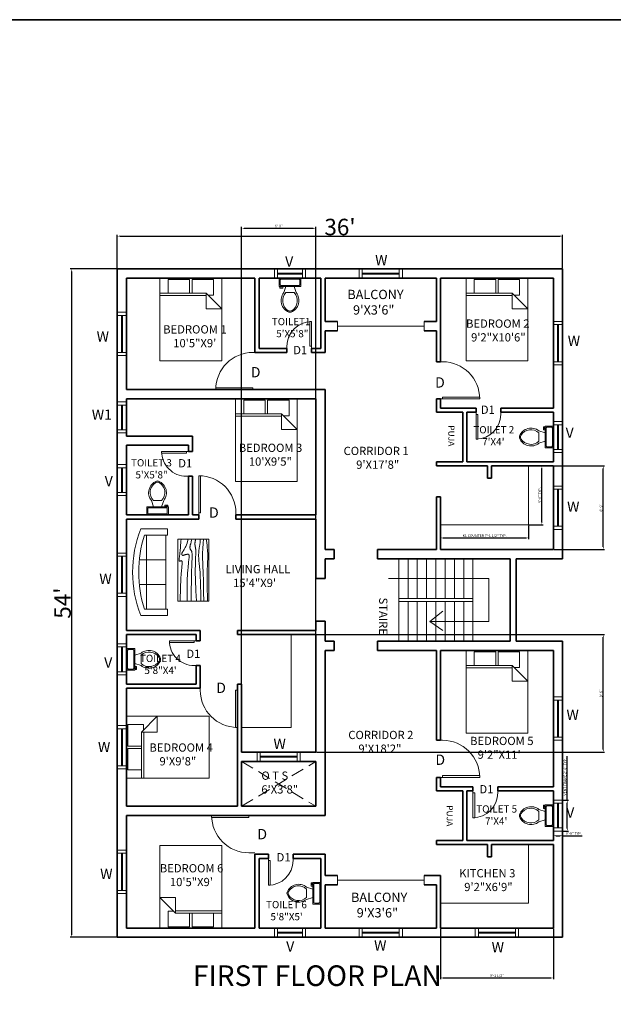
# Model space of a CAD drawing. Units: inches. Extents: x 2391 to 16591, y 7259 to 10239.
# Tile 20 of 27: x 2970 to 3545, y 9285 to 10239. Entities that reach past the tile are written whole.
import ezdxf

# ---------------------------------------------------------------- set-up
doc = ezdxf.new("R2010")
doc.units = ezdxf.units.IN
doc.linetypes.add('DASHED', pattern=[19.05, 12.7, -6.35])
for name, color, linetype, lineweight in [('A-ANNO-DIMS', 4, 'Continuous', 18), ('A-ANNO-IDEN', 2, 'Continuous', 18), ('A-ANNO-SYMB', 3, 'Continuous', 18), ('A-ANNO-TITL', 3, 'Continuous', 30), ('A-ANNO-TTLB', 7, 'Continuous', 35), ('A-AREA-IDEN', 7, 'Continuous', 18), ('A-DOOR', 3, 'Continuous', 18), ('A-FLOR-CASE', 6, 'Continuous', 18), ('A-FLOR-FIXT', 9, 'Continuous', 18), ('A-FLOR-HRAL', 8, 'Continuous', 18), ('A-FLOR-OPEN', 4, 'DASHED', 13), ('A-FLOR-STRS', 7, 'Continuous', 18), ('A-FURN', 8, 'Continuous', 18), ('A-GLAZ', 4, 'Continuous', 18), ('A-WALL', 7, 'Continuous', 35)]:
    doc.layers.add(name, color=color, linetype=linetype, lineweight=lineweight)
doc.styles.get("Standard").update_dxf_attribs({"font": 'arial.ttf'})
doc.dimstyles.new('ISO-25', dxfattribs={"dimtxt": 2.5, "dimasz": 2.5, "dimexe": 1.25, "dimexo": 0.625, "dimtad": 1, "dimdec": 0, "dimlunit": 3, "dimtxsty": 'Standard', "dimcen": 2.5, "dimadec": 0, "dimazin": 0, "dimtfac": 1, "dimtdec": 0, "dimtmove": 0, "dimatfit": 3, "dimfxl": 1, "dimarcsym": 0})

# ---------------------------------------------------------------- blocks, each defined once
blk = doc.blocks.new('Bed - Queen')
for p, q in [((0, -80.00003), (0, 0)), ((0, 0), (59.99999, 0)), ((59.99999, 0), (59.99999, -80.00003)), ((7.99999, -1.2), (28.79998, -1.2)), ((7.99999, -14.4), (7.99999, -1.2)), ((28.79998, -1.2), (28.79998, -14.4)), ((31.19999, -1.2), (51.99999, -1.2)), ((31.19999, -14.4), (31.19999, -1.2)), ((51.99999, -1.2), (51.99999, -16.4)), ((0, -14.4), (44.8, -14.4)), ((44.8, -16.8), (0, -16.8)), ((59.99999, -29.6), (44.8, -14.4)), ((44.8, -14.4), (44.8, -29.6)), ((51.99999, -16.4), (46.79936, -16.4)), ((44.8, -29.6), (59.99999, -29.6)), ((59.99999, -80.00003), (0, -80.00003))]:
    blk.add_line(p, q)
blk = doc.blocks.new('Sofa - Roundback 7 ft.')
for p, q in [((-12.00002, -32.4421), (-12.00003, -6.5971)), ((11.99997, -32.4421), (11.99998, -6.5971)), ((-36.000027, -34), (-36.000027, -11.4696)), ((-35.999844, -13.3819), (35.9998, -13.3819)), ((35.99998, -34), (35.99998, -11.4696)), ((-36.000027, -32.4421), (35.99998, -32.4421))]:
    blk.add_line(p, q)
for points in [[(-36.000027, -34), (-42.000027, -34), (-42.000027, -8)], [(41.99998, -8), (41.99998, -34), (35.99998, -34)]]:
    blk.add_lwpolyline(points)
for centre, radius, start, end in [((0, -114.25), 114.25, 68.43141, 111.5686), ((-0.00001, -127.1968), 121.1968, 72.72033, 107.2797)]:
    blk.add_arc(centre, radius, start, end)
blk = doc.blocks.new('Table - Rectangular Woodgrain 60 x 30 in.')
for p, q in [((0, 0), (0, -30)), ((60, 0), (0, 0)), ((60, -30), (60, 0)), ((0, -30), (60, -30))]:
    blk.add_line(p, q)
for points in [[(0, -2.4), (4.8155, -2.418), (9.0302, -2.4688), (12.709, -2.5477), (15.9167, -2.65), (18.7181, -2.7711), (21.1781, -2.9063), (23.3616, -3.0508), (25.3333, -3.2), (27.1477, -3.3495), (28.8172, -3.4958), (30.3437, -3.636), (31.7291, -3.7667), (32.9756, -3.8849), (34.0849, -3.9875), (35.059, -4.0714), (35.9, -4.1334), (36.6114, -4.1711), (37.2041, -4.1854), (37.6906, -4.1779), (38.0833, -4.15), (38.3948, -4.1034), (38.6375, -4.0396), (38.8239, -3.9602), (38.9666, -3.8667), (39.0764, -3.7608), (39.1573, -3.6448), (39.2116, -3.521), (39.2416, -3.3917), (39.2498, -3.2593), (39.2385, -3.1261), (39.21, -2.9944), (39.1666, -2.8667), (39.111, -2.7447), (39.0468, -2.6281), (38.978, -2.5163), (38.9083, -2.4083), (38.8418, -2.3035), (38.7823, -2.201), (38.7337, -2.1001), (38.7, -2), (38.6844, -1.9003), (38.6875, -1.8021), (38.7094, -1.707), (38.75, -1.6167), (38.8094, -1.5326), (38.8875, -1.4563), (38.9844, -1.3893), (39.1, -1.3333), (39.2351, -1.2896), (39.3937, -1.2583), (39.5804, -1.2396), (39.8, -1.2333), (40.057, -1.2396), (40.3562, -1.2583), (40.7023, -1.2896), (41.1, -1.3333), (41.5547, -1.3895), (42.0755, -1.4573), (42.6721, -1.5361), (43.3542, -1.625), (44.1316, -1.7233), (45.014, -1.8302), (46.0114, -1.9449), (47.1333, -2.0667), (48.3862, -2.1947), (49.7625, -2.3281), (51.2513, -2.4663), (52.8416, -2.6083), (54.5226, -2.7535), (56.2833, -2.9011), (58.1127, -3.0501), (60, -3.2)], [(0, -9.2), (6.5759, -9.0858), (11.9385, -9.0365), (16.2527, -9.0418), (19.6833, -9.0917), (22.3952, -9.1759), (24.5531, -9.2844), (26.322, -9.4069), (27.8666, -9.5333), (29.3241, -9.6553), (30.7203, -9.7719), (32.0532, -9.8837), (33.3208, -9.9917), (34.5213, -10.0965), (35.6526, -10.199), (36.7128, -10.2999), (37.7, -10.4), (38.6129, -10.4996), (39.4531, -10.5969), (40.223, -10.6895), (40.925, -10.775), (41.5613, -10.8512), (42.1344, -10.9156), (42.6465, -10.966), (43.1, -11), (43.4976, -11.0158), (43.8437, -11.0136), (44.143, -10.9942), (44.4, -10.9583), (44.6195, -10.9069), (44.8062, -10.8406), (44.9648, -10.7603), (45.1, -10.6667), (45.2155, -10.5598), (45.3114, -10.4365), (45.3871, -10.2929), (45.4416, -10.125), (45.4743, -9.929), (45.4844, -9.7011), (45.4709, -9.4371), (45.4333, -9.1333), (45.3716, -8.7883), (45.2896, -8.4104), (45.1919, -8.0107), (45.0833, -7.6), (44.9685, -7.1893), (44.8521, -6.7896), (44.7388, -6.4117), (44.6333, -6.0667), (44.54, -5.7628), (44.4614, -5.4979), (44.4001, -5.2675), (44.3583, -5.0667), (44.3384, -4.8909), (44.3427, -4.7354), (44.3736, -4.5956), (44.4333, -4.4667), (44.5236, -4.3453), (44.6427, -4.2333), (44.7884, -4.1339), (44.9583, -4.05), (45.1501, -3.9849), (45.3614, -3.9417), (45.59, -3.9234), (45.8333, -3.9333), (46.0915, -3.9749), (46.3734, -4.0531), (46.6906, -4.1736), (47.0542, -4.3417), (47.4756, -4.5629), (47.9661, -4.8427), (48.5372, -5.1866), (49.2, -5.6), (49.9676, -6.0844), (50.8594, -6.625), (51.8965, -7.2031), (53.1, -7.8), (54.491, -8.3969), (56.0906, -8.975), (57.9199, -9.5156), (60, -10)], [(0, -12.8), (5.1847, -12.9322), (9.6213, -13.0323), (13.3963, -13.1059), (16.5958, -13.1583), (19.3063, -13.1952), (21.614, -13.2219), (23.6054, -13.2439), (25.3666, -13.2667), (26.9728, -13.2947), (28.4531, -13.3281), (29.8256, -13.3663), (31.1083, -13.4083), (32.3191, -13.4535), (33.476, -13.501), (34.597, -13.5501), (35.7, -13.6), (36.7984, -13.6497), (37.8875, -13.6979), (38.9578, -13.743), (40, -13.7833), (41.0047, -13.8174), (41.9625, -13.8438), (42.864, -13.8607), (43.7, -13.8667), (44.4631, -13.8604), (45.1552, -13.8417), (45.7801, -13.8104), (46.3416, -13.7667), (46.8439, -13.7104), (47.2906, -13.6417), (47.6858, -13.5604), (48.0333, -13.4667), (48.3375, -13.3608), (48.6042, -13.2448), (48.8396, -13.121), (49.05, -12.9917), (49.2417, -12.8593), (49.4208, -12.7261), (49.5937, -12.5944), (49.7667, -12.4667), (49.9452, -12.3451), (50.1323, -12.2313), (50.3303, -12.1268), (50.5416, -12.0333), (50.7686, -11.9524), (51.0135, -11.8854), (51.2788, -11.8341), (51.5666, -11.8), (51.8785, -11.7843), (52.2116, -11.7865), (52.562, -11.8059), (52.926, -11.8417), (53.2998, -11.8931), (53.6795, -11.9594), (54.0614, -12.0397), (54.4416, -12.1333), (54.8223, -12.2401), (55.2293, -12.3625), (55.6942, -12.5037), (56.2489, -12.6667), (56.9251, -12.8547), (57.7545, -13.0708), (58.7689, -13.3182), (60, -13.6)], [(0, -18), (5.124, -17.7273), (9.6609, -17.5057), (13.6705, -17.3303), (17.2125, -17.1958), (20.3467, -17.0973), (23.1328, -17.0297), (25.6307, -16.9878), (27.9, -16.9667), (29.9928, -16.9617), (31.9302, -16.9703), (33.7254, -16.9907), (35.3917, -17.0208), (36.9423, -17.0588), (38.3906, -17.1026), (39.7499, -17.1503), (41.0333, -17.2), (42.2519, -17.2496), (43.4073, -17.2969), (44.4986, -17.3395), (45.525, -17.375), (46.4858, -17.4012), (47.3802, -17.4156), (48.2074, -17.416), (48.9667, -17.4), (49.6583, -17.3662), (50.2872, -17.3167), (50.8595, -17.2547), (51.3812, -17.1833), (51.8584, -17.1057), (52.2971, -17.025), (52.7034, -16.9443), (53.0833, -16.8667), (53.443, -16.7951), (53.789, -16.7313), (54.128, -16.6768), (54.4666, -16.6334), (54.8115, -16.6024), (55.1693, -16.5854), (55.5465, -16.5841), (55.95, -16.6), (56.3828, -16.6337), (56.8346, -16.6823), (57.2915, -16.7418), (57.7396, -16.8084), (58.165, -16.878), (58.5539, -16.9469), (58.8924, -17.0111), (59.1666, -17.0667), (59.3679, -17.1107), (59.5078, -17.1438), (59.6032, -17.1675), (59.6708, -17.1833), (59.7275, -17.193), (59.7901, -17.1979), (59.8753, -17.1998), (60, -17.2)], [(0, -22.4), (8.0098, -22.2501), (14.4094, -22.1011), (19.4168, -21.9535), (23.25, -21.8083), (26.1269, -21.6663), (28.2656, -21.5281), (29.884, -21.3947), (31.2, -21.2667), (32.3967, -21.1448), (33.5172, -21.0292), (34.5697, -20.9198), (35.5625, -20.8167), (36.5037, -20.7198), (37.4015, -20.6292), (38.2642, -20.5448), (39.1, -20.4667), (39.9164, -20.3951), (40.7187, -20.3313), (41.5117, -20.2768), (42.3, -20.2333), (43.0883, -20.2024), (43.8812, -20.1854), (44.6836, -20.1841), (45.5, -20.2), (46.3328, -20.234), (47.1747, -20.2844), (48.0163, -20.3488), (48.8479, -20.425), (49.66, -20.5106), (50.4429, -20.6031), (51.1872, -20.7004), (51.8833, -20.8), (52.5246, -20.8999), (53.1166, -20.9995), (53.6681, -21.0983), (54.1875, -21.1958), (54.6834, -21.2919), (55.1646, -21.3859), (55.6394, -21.4777), (56.1167, -21.5667), (56.6028, -21.6515), (57.0961, -21.7266), (57.5929, -21.7852), (58.0896, -21.8208), (58.5823, -21.8268), (59.0674, -21.7964), (59.5412, -21.723), (60, -21.6)], [(0, -25.2), (8.6355, -25.0504), (15.7026, -24.9031), (21.4049, -24.7606), (25.9458, -24.625), (29.529, -24.4988), (32.3578, -24.3844), (34.6359, -24.284), (36.5667, -24.2), (38.3213, -24.1341), (39.9417, -24.0854), (41.437, -24.0523), (42.8167, -24.0333), (44.0901, -24.0268), (45.2667, -24.0313), (46.3557, -24.0451), (47.3667, -24.0667), (48.309, -24.0947), (49.1928, -24.1287), (50.0284, -24.168), (50.826, -24.2125), (51.5959, -24.2617), (52.3483, -24.3151), (53.0935, -24.3725), (53.8417, -24.4334), (54.6009, -24.497), (55.3699, -24.561), (56.1454, -24.6226), (56.9239, -24.6792), (57.7021, -24.7279), (58.4764, -24.7662), (59.2435, -24.7911), (60, -24.8)], [(0, -28.8), (5.6867, -28.6681), (10.45, -28.5698), (14.407, -28.5012), (17.675, -28.4584), (20.3711, -28.4374), (22.6125, -28.4344), (24.5164, -28.4455), (26.2, -28.4667), (27.762, -28.4947), (29.2276, -28.5281), (30.6033, -28.5663), (31.8958, -28.6084), (33.1118, -28.6535), (34.2578, -28.7011), (35.3405, -28.7501), (36.3666, -28.8), (37.3443, -28.8497), (38.288, -28.8974), (39.2137, -28.9412), (40.1375, -28.9792), (41.0753, -29.0093), (42.0432, -29.0297), (43.0572, -29.0384), (44.1333, -29.0333), (45.2936, -29.0114), (46.5843, -28.9641), (48.0579, -28.8816), (49.7666, -28.7542), (51.7629, -28.5721), (54.0989, -28.3255), (56.8272, -28.0048), (60, -27.6)]]:
    blk.add_lwpolyline(points)
blk = doc.blocks.new('Toilet - top')
for p, q in [((-10, -8.5), (-8, -8.5)), ((-10, -9.5), (-10, -8.5)), ((-7, -9.5), (-10, -9.5)), ((-8, -8.5), (-8, -8)), ((-7, -8), (-7, -9.5)), ((-4, -8), (-6, -14)), ((4, -8), (6, -14)), ((9.5, -6), (9.5, -2)), ((4, -14), (-4, -14))]:
    blk.add_line(p, q)
blk.add_lwpolyline([(10.5, -8), (10.5, 0), (-10.5, 0), (-10.5, -8)], close=True)
for points in [[(-9.5, -2), (-9.5, -6)], [(8.5, -1), (-8.5, -1)], [(-8.5, -7), (8.5, -7)]]:
    blk.add_lwpolyline(points)
for centre, radius, start, end in [((-8.62, -1.88), 0.884, 81.8699, 188.1301), ((-8.62, -6.12), 0.884, 171.8699, 278.1301), ((8.62, -1.88), 0.884, 351.8699, 98.1301), ((8.62, -6.12), 0.884, 261.8699, 8.1301), ((3.52, -21.58), 12.17, 141.46911, 247.97143), ((4.2, -21.82), 11.33, 136.36773, 238.94682), ((-3.52, -21.58), 12.17, 292.02843, 38.53071), ((-4.2, -21.82), 11.33, 301.05301, 43.63209), ((0, -27.88), 4, 245.73182, 294.26817), ((0, -29), 4, 254.86053, 285.13947)]:
    blk.add_arc(centre, radius, start, end)
blk = doc.blocks.new('*U11')
for p, q in [((-36, 0), (-36, 6)), ((0, 0), (0, 6))]:
    blk.add_line(p, q)
blk.add_lwpolyline([(0, 0), (0, -36), (-1.75, -36), (-1.75, 0)], close=True)
blk.add_arc((0, 0), 36, 180, 270)
blk = doc.blocks.new('*U8')
for p, q in [((-24, 0), (-24, -6)), ((0, 0), (0, -6))]:
    blk.add_line(p, q)
blk.add_lwpolyline([(0, 0), (0, 24), (-1.75, 24), (-1.75, 0)], close=True)
blk.add_arc((0, 0), 24, 90, 180)
blk = doc.blocks.new('*U12')
for p, q in [((0, 0), (0, -6)), ((-36, 0), (-36, -6))]:
    blk.add_line(p, q)
blk.add_lwpolyline([(0, 0), (0, 36), (-1.75, 36), (-1.75, 0)], close=True)
blk.add_arc((0, 0), 36, 90, 180)
blk = doc.blocks.new('*U9')
for p, q in [((0, 0), (0, 6)), ((24, 0), (24, 6))]:
    blk.add_line(p, q)
blk.add_lwpolyline([(0, 0), (0, -24), (1.75, -24), (1.75, 0)], close=True)
blk.add_arc((0, 0), 24, 270, 0)
blk = doc.blocks.new('*U7')
for p, q in [((0, 0), (0, -6)), ((36, 0), (36, -6))]:
    blk.add_line(p, q)
blk.add_lwpolyline([(0, 0), (0, 36), (1.75, 36), (1.75, 0)], close=True)
blk.add_arc((0, 0), 36, 0, 90)
blk = doc.blocks.new('*U6')
for p, q in [((-36, 0), (-36, 6)), ((0, 0), (0, 6))]:
    blk.add_line(p, q)
blk.add_lwpolyline([(0, 0), (0, -36), (-1.75, -36), (-1.75, 0)], close=True)
blk.add_arc((0, 0), 36, 180, 270)
blk = doc.blocks.new('*U13')
for p, q in [((0, 0), (0, 6)), ((36, 0), (36, 6))]:
    blk.add_line(p, q)
blk.add_lwpolyline([(0, 0), (0, -36), (1.75, -36), (1.75, 0)], close=True)
blk.add_arc((0, 0), 36, 270, 0)
blk = doc.blocks.new('*U10')
for p, q in [((0, 0), (0, -6)), ((-36, 0), (-36, -6))]:
    blk.add_line(p, q)
blk.add_lwpolyline([(0, 0), (0, 36), (-1.75, 36), (-1.75, 0)], close=True)
blk.add_arc((0, 0), 36, 90, 180)
blk = doc.blocks.new('*D16')
at = {"layer": 'A-ANNO-DIMS', "color": 0, "lineweight": -2, "transparency": 16777216}
for p, q in [((3064.34, 9998.38), (3064.34, 10030.84)), ((3066.84, 10029.59), (3493.84, 10029.59)), ((3496.34, 9998.38), (3496.34, 10030.84))]:
    blk.add_line(p, q, dxfattribs=at)
at = {"layer": 'A-ANNO-DIMS', "color": 0, "transparency": 16777216}
for points in [[(3066.84, 10030), (3066.84, 10029.17), (3064.34, 10029.59)], [(3493.84, 10030), (3493.84, 10029.17), (3496.34, 10029.59)]]:
    blk.add_solid(points, dxfattribs=at)
at = {"layer": 'Defpoints', "color": 0, "transparency": 16777216}
for p in [(3496.34, 10029.59), (3064.34, 9997.76), (3496.34, 9997.76)]:
    blk.add_point(p, dxfattribs=at)
at = {"layer": 'A-ANNO-DIMS', "color": 0, "transparency": 16777216, "insert": (3280.34, 10038.39), "char_height": 2.5, "attachment_point": 5}
blk.add_mtext("{\\H6.4x;36'}", dxfattribs=at)
blk = doc.blocks.new('*D17')
at = {"layer": 'A-ANNO-DIMS', "color": 0, "lineweight": -2, "transparency": 16777216}
for p, q in [((3063.71, 9997.76), (3018.73, 9997.76)), ((3019.98, 9995.26), (3019.98, 9352.26)), ((3063.71, 9349.76), (3018.73, 9349.76))]:
    blk.add_line(p, q, dxfattribs=at)
at = {"layer": 'A-ANNO-DIMS', "color": 0, "transparency": 16777216}
for points in [[(3019.56, 9995.26), (3020.39, 9995.26), (3019.98, 9997.76)], [(3019.56, 9352.26), (3020.39, 9352.26), (3019.98, 9349.76)]]:
    blk.add_solid(points, dxfattribs=at)
at = {"layer": 'Defpoints', "color": 0, "transparency": 16777216}
for p in [(3064.34, 9997.76), (3019.98, 9349.76), (3064.34, 9349.76)]:
    blk.add_point(p, dxfattribs=at)
at = {"layer": 'A-ANNO-DIMS', "color": 0, "transparency": 16777216, "insert": (3011.22, 9673.76), "char_height": 2.5, "attachment_point": 5, "rotation": 90}
blk.add_mtext("{\\H6.4x;54'}", dxfattribs=at)
blk = doc.blocks.new('WINDOW-36-PLAN')
for p, q in [((9, 42), (0, 42)), ((9, 39), (0, 39)), ((4, 39), (4, 3)), ((4.5, 39), (4.5, 3)), ((5, 39), (5, 3)), ((9, 3), (0, 3)), ((9, 0), (0, 0))]:
    blk.add_line(p, q)
blk = doc.blocks.new('VENT-24-PLAN')
for p, q in [((9, 30), (0, 30)), ((9, 27), (0, 27)), ((4, 27), (4, 3)), ((4.5, 27), (4.5, 3)), ((5, 27), (5, 3)), ((9, 3), (0, 3)), ((9, 0), (0, 0))]:
    blk.add_line(p, q)
blk = doc.blocks.new('WINDOW-24-PLAN')
for p, q in [((9, 30), (0, 30)), ((9, 27), (0, 27)), ((4, 27), (4, 3)), ((4.5, 27), (4.5, 3)), ((5, 27), (5, 3)), ((9, 3), (0, 3)), ((9, 0), (0, 0))]:
    blk.add_line(p, q)
blk = doc.blocks.new('STAIR-RETURN-FLIGHT')
for p, q in [((0, 80), (0, 0)), ((9, 80), (9, 41.5)), ((18, 80), (18, 41.5)), ((27, 80), (27, 41.5)), ((36, 80), (36, 41.5)), ((45, 80), (45, 41.5)), ((54, 80), (54, 41.5)), ((63, 80), (63, 41.5)), ((72, 80), (72, 0)), ((72, 41.5), (0, 41.5)), ((72, 38.5), (0, 38.5)), ((9, 38.5), (9, 0)), ((18, 38.5), (18, 0)), ((27, 38.5), (27, 0)), ((36, 38.5), (36, 0)), ((45, 38.5), (45, 0)), ((54, 38.5), (54, 0)), ((63, 38.5), (63, 0))]:
    blk.add_line(p, q)
blk = doc.blocks.new('STAIR-DIRECTION-ARROW')
for p, q in [((0, 50.31), (97.37, 50.31)), ((97.37, 50.31), (97.37, 8.81)), ((40.34, 8.81), (52.74, 18.89)), ((97.37, 8.81), (40.34, 8.81)), ((40.34, 8.81), (52.74, 0))]:
    blk.add_line(p, q)
blk = doc.blocks.new('COUNTER-L-KITCHEN')
for p, q in [((85.5, 57), (85.5, 0)), ((85.5, 0), (0, 0))]:
    blk.add_line(p, q)
blk = doc.blocks.new('*D43')
at = {"layer": 'A-ANNO-DIMS', "color": 0, "lineweight": -2, "transparency": 16777216}
for p, q in [((3500.84, 9482.76), (3500.84, 9525.35)), ((3496.96, 9482.76), (3502.09, 9482.76)), ((3500.84, 9455.26), (3500.84, 9480.26)), ((3496.96, 9452.76), (3502.09, 9452.76))]:
    blk.add_line(p, q, dxfattribs=at)
at = {"layer": 'A-ANNO-DIMS', "color": 0, "transparency": 16777216}
for points in [[(3500.42, 9480.26), (3501.26, 9480.26), (3500.84, 9482.76)], [(3500.42, 9455.26), (3501.26, 9455.26), (3500.84, 9452.76)]]:
    blk.add_solid(points, dxfattribs=at)
at = {"layer": 'Defpoints', "color": 0, "transparency": 16777216}
for p in [(3496.34, 9482.76), (3500.84, 9482.76), (3496.34, 9452.76)]:
    blk.add_point(p, dxfattribs=at)
at = {"layer": 'A-ANNO-DIMS', "color": 0, "transparency": 16777216, "insert": (3498.94, 9505.31), "char_height": 2.5, "attachment_point": 5, "rotation": 90}
blk.add_mtext('VENT FRAME 2\'-6" TYP.', dxfattribs=at)
blk = doc.blocks.new('*D44')
at = {"layer": 'A-ANNO-DIMS', "color": 0, "lineweight": -2, "transparency": 16777216}
for p, q in [((3487.34, 9452.13), (3487.34, 9447.01)), ((3496.34, 9452.13), (3496.34, 9447.01)), ((3489.84, 9448.26), (3493.84, 9448.26)), ((3496.34, 9448.26), (3515.33, 9448.26))]:
    blk.add_line(p, q, dxfattribs=at)
at = {"layer": 'A-ANNO-DIMS', "color": 0, "transparency": 16777216}
for points in [[(3489.84, 9448.67), (3489.84, 9447.84), (3487.34, 9448.26)], [(3493.84, 9448.67), (3493.84, 9447.84), (3496.34, 9448.26)]]:
    blk.add_solid(points, dxfattribs=at)
at = {"layer": 'Defpoints', "color": 0, "transparency": 16777216}
for p in [(3487.34, 9452.76), (3496.34, 9452.76), (3496.34, 9448.26)]:
    blk.add_point(p, dxfattribs=at)
at = {"layer": 'A-ANNO-DIMS', "color": 0, "transparency": 16777216, "insert": (3507.08, 9450.16), "char_height": 2.5, "attachment_point": 5}
blk.add_mtext('0\'-9" TYP.', dxfattribs=at)
blk = doc.blocks.new('*D53')
at = {"layer": 'A-ANNO-DIMS', "color": 0, "lineweight": -2, "transparency": 16777216}
for p, q in [((3377.84, 9749.13), (3377.84, 9735.68)), ((3463.34, 9749.13), (3463.34, 9735.68)), ((3380.34, 9736.93), (3460.84, 9736.93))]:
    blk.add_line(p, q, dxfattribs=at)
at = {"layer": 'A-ANNO-DIMS', "color": 0, "transparency": 16777216}
for points in [[(3380.34, 9737.35), (3380.34, 9736.52), (3377.84, 9736.93)], [(3460.84, 9737.35), (3460.84, 9736.52), (3463.34, 9736.93)]]:
    blk.add_solid(points, dxfattribs=at)
at = {"layer": 'Defpoints', "color": 0, "transparency": 16777216}
for p in [(3377.84, 9749.76), (3463.34, 9749.76), (3463.34, 9736.93)]:
    blk.add_point(p, dxfattribs=at)
at = {"layer": 'A-ANNO-DIMS', "color": 0, "transparency": 16777216, "insert": (3420.59, 9738.85), "char_height": 2.5, "attachment_point": 5}
blk.add_mtext('K1 COUNTER 7\'-1 1/2" TYP.', dxfattribs=at)
blk = doc.blocks.new('*D54')
at = {"layer": 'A-ANNO-DIMS', "color": 0, "lineweight": -2, "transparency": 16777216}
for p, q in [((3463.96, 9806.76), (3477.41, 9806.76)), ((3476.16, 9752.26), (3476.16, 9804.26)), ((3463.96, 9749.76), (3477.41, 9749.76))]:
    blk.add_line(p, q, dxfattribs=at)
at = {"layer": 'A-ANNO-DIMS', "color": 0, "transparency": 16777216}
for points in [[(3475.75, 9804.26), (3476.58, 9804.26), (3476.16, 9806.76)], [(3475.75, 9752.26), (3476.58, 9752.26), (3476.16, 9749.76)]]:
    blk.add_solid(points, dxfattribs=at)
at = {"layer": 'Defpoints', "color": 0, "transparency": 16777216}
for p in [(3463.34, 9806.76), (3476.16, 9806.76), (3463.34, 9749.76)]:
    blk.add_point(p, dxfattribs=at)
at = {"layer": 'A-ANNO-DIMS', "color": 0, "transparency": 16777216, "insert": (3474.26, 9778.26), "char_height": 2.5, "attachment_point": 5, "rotation": 90}
blk.add_mtext('4\'-9" TYP.', dxfattribs=at)
blk = doc.blocks.new('*D74')
at = {"layer": 'A-ANNO-DIMS', "color": 0, "lineweight": -2, "transparency": 16777216}
for p, q in [((3377.84, 9358.13), (3377.84, 9309.11)), ((3487.34, 9358.13), (3487.34, 9309.11)), ((3380.34, 9310.36), (3484.84, 9310.36))]:
    blk.add_line(p, q, dxfattribs=at)
at = {"layer": 'A-ANNO-DIMS', "color": 0, "transparency": 16777216}
for points in [[(3380.34, 9310.77), (3380.34, 9309.94), (3377.84, 9310.36)], [(3484.84, 9310.77), (3484.84, 9309.94), (3487.34, 9310.36)]]:
    blk.add_solid(points, dxfattribs=at)
at = {"layer": 'Defpoints', "color": 0, "transparency": 16777216}
for p in [(3377.84, 9358.76), (3487.34, 9358.76), (3487.34, 9310.36)]:
    blk.add_point(p, dxfattribs=at)
at = {"layer": 'A-ANNO-DIMS', "color": 0, "transparency": 16777216, "insert": (3432.59, 9312.28), "char_height": 2.5, "attachment_point": 5}
blk.add_mtext('9\'-1 1/2"', dxfattribs=at)
blk = doc.blocks.new('*D75')
at = {"layer": 'A-ANNO-DIMS', "color": 0, "lineweight": -2, "transparency": 16777216}
for p, q in [((3487.96, 9806.76), (3536.99, 9806.76)), ((3535.74, 9728.26), (3535.74, 9804.26)), ((3487.96, 9725.76), (3536.99, 9725.76))]:
    blk.add_line(p, q, dxfattribs=at)
at = {"layer": 'A-ANNO-DIMS', "color": 0, "transparency": 16777216}
for points in [[(3535.32, 9804.26), (3536.16, 9804.26), (3535.74, 9806.76)], [(3535.32, 9728.26), (3536.16, 9728.26), (3535.74, 9725.76)]]:
    blk.add_solid(points, dxfattribs=at)
at = {"layer": 'Defpoints', "color": 0, "transparency": 16777216}
for p in [(3487.34, 9806.76), (3535.74, 9806.76), (3487.34, 9725.76)]:
    blk.add_point(p, dxfattribs=at)
at = {"layer": 'A-ANNO-DIMS', "color": 0, "transparency": 16777216, "insert": (3533.84, 9766.26), "char_height": 2.5, "attachment_point": 5, "rotation": 90}
blk.add_mtext('6\'-9"', dxfattribs=at)
blk = doc.blocks.new('*D76')
at = {"layer": 'A-ANNO-DIMS', "color": 0, "lineweight": -2, "transparency": 16777216}
for p, q in [((3184.84, 9529.88), (3184.84, 10038.41)), ((3187.34, 10037.16), (3254.34, 10037.16)), ((3256.84, 9529.88), (3256.84, 10038.41))]:
    blk.add_line(p, q, dxfattribs=at)
at = {"layer": 'A-ANNO-DIMS', "color": 0, "transparency": 16777216}
for points in [[(3187.34, 10037.57), (3187.34, 10036.74), (3184.84, 10037.16)], [(3254.34, 10037.57), (3254.34, 10036.74), (3256.84, 10037.16)]]:
    blk.add_solid(points, dxfattribs=at)
at = {"layer": 'Defpoints', "color": 0, "transparency": 16777216}
for p in [(3256.84, 10037.16), (3184.84, 9529.26), (3256.84, 9529.26)]:
    blk.add_point(p, dxfattribs=at)
at = {"layer": 'A-ANNO-DIMS', "color": 0, "transparency": 16777216, "insert": (3220.84, 10039.06), "char_height": 2.5, "attachment_point": 5}
blk.add_mtext('6\'-0"', dxfattribs=at)
blk = doc.blocks.new('*D77')
at = {"layer": 'A-ANNO-DIMS', "color": 0, "lineweight": -2, "transparency": 16777216}
for p, q in [((3257.46, 9643.26), (3536.99, 9643.26)), ((3535.74, 9531.76), (3535.74, 9640.76)), ((3257.46, 9529.26), (3536.99, 9529.26))]:
    blk.add_line(p, q, dxfattribs=at)
at = {"layer": 'A-ANNO-DIMS', "color": 0, "transparency": 16777216}
for points in [[(3535.32, 9640.76), (3536.16, 9640.76), (3535.74, 9643.26)], [(3535.32, 9531.76), (3536.16, 9531.76), (3535.74, 9529.26)]]:
    blk.add_solid(points, dxfattribs=at)
at = {"layer": 'Defpoints', "color": 0, "transparency": 16777216}
for p in [(3256.84, 9643.26), (3535.74, 9643.26), (3256.84, 9529.26)]:
    blk.add_point(p, dxfattribs=at)
at = {"layer": 'A-ANNO-DIMS', "color": 0, "transparency": 16777216, "insert": (3533.84, 9586.26), "char_height": 2.5, "attachment_point": 5, "rotation": 90}
blk.add_mtext('9\'-6"', dxfattribs=at)

msp = doc.modelspace()

# ---------------------------------------------------------------- linework, layer by layer
at = {"layer": 'A-ANNO-TTLB'}
msp.add_lwpolyline([(2391.28, 10239.38), (4154.2, 10239.38), (4154.2, 7258.54), (2391.28, 7258.54)], close=True, dxfattribs=at)
at = {"layer": 'A-FLOR-CASE'}
for p, q in [((3232.84, 9553.26), (3232.84, 9643.26)), ((3184.84, 9553.26), (3232.84, 9553.26))]:
    msp.add_line(p, q, dxfattribs=at)
at = {"layer": 'A-FLOR-HRAL'}
for p, q in [((3277.84, 9937.76), (3277.84, 9946.76)), ((3361.84, 9937.76), (3361.84, 9946.76)), ((3277.84, 9942.26), (3361.84, 9942.26)), ((3277.84, 9400.76), (3277.84, 9409.76)), ((3277.84, 9405.26), (3361.84, 9405.26)), ((3361.84, 9400.76), (3361.84, 9409.76))]:
    msp.add_line(p, q, dxfattribs=at)
at = {"layer": 'A-FLOR-OPEN'}
for p, q in [((3184.84, 9476.76), (3256.84, 9520.26)), ((3184.84, 9520.26), (3256.84, 9476.76))]:
    msp.add_line(p, q, dxfattribs=at)
at = {"layer": 'A-WALL'}
for p, q in [((3064.34, 9997.76), (3496.34, 9997.76)), ((3064.34, 9349.76), (3064.34, 9997.76)), ((3496.34, 9997.76), (3496.34, 9716.76)), ((3073.34, 9988.76), (3197.84, 9988.76)), ((3073.34, 9880.76), (3073.34, 9988.76)), ((3197.84, 9916.76), (3197.84, 9988.76)), ((3201.84, 9920.76), (3201.84, 9988.76)), ((3201.84, 9988.76), (3261.84, 9988.76)), ((3261.84, 9920.76), (3261.84, 9988.76)), ((3265.84, 9946.76), (3265.84, 9988.76)), ((3265.84, 9988.76), (3373.84, 9988.76)), ((3373.84, 9946.76), (3373.84, 9988.76)), ((3377.84, 9907.76), (3377.84, 9988.76)), ((3377.84, 9988.76), (3487.34, 9988.76)), ((3487.34, 9988.76), (3487.34, 9862.76)), ((3265.84, 9946.76), (3277.84, 9946.76)), ((3361.84, 9946.76), (3373.84, 9946.76)), ((3265.84, 9937.76), (3277.84, 9937.76)), ((3265.84, 9916.76), (3265.84, 9937.76)), ((3361.84, 9937.76), (3373.84, 9937.76)), ((3373.84, 9907.76), (3373.84, 9937.76)), ((3201.84, 9920.76), (3228.84, 9920.76)), ((3228.84, 9916.76), (3228.84, 9920.76)), ((3252.84, 9916.76), (3252.84, 9920.76)), ((3252.84, 9920.76), (3261.84, 9920.76)), ((3197.84, 9916.76), (3228.84, 9916.76)), ((3252.84, 9916.76), (3265.84, 9916.76)), ((3373.84, 9907.76), (3377.84, 9907.76)), ((3073.34, 9880.76), (3265.84, 9880.76)), ((3265.84, 9725.76), (3265.84, 9880.76)), ((3073.34, 9871.76), (3256.84, 9871.76)), ((3073.34, 9835.76), (3073.34, 9871.76)), ((3256.84, 9759.26), (3256.84, 9871.76)), ((3373.84, 9858.76), (3373.84, 9871.76)), ((3373.84, 9871.76), (3377.84, 9871.76)), ((3377.84, 9862.76), (3377.84, 9871.76)), ((3377.84, 9862.76), (3412.34, 9862.76)), ((3412.34, 9862.76), (3412.34, 9858.76)), ((3436.34, 9862.76), (3436.34, 9858.76)), ((3436.34, 9862.76), (3487.34, 9862.76)), ((3373.84, 9858.76), (3399.34, 9858.76)), ((3399.34, 9858.76), (3399.34, 9810.76)), ((3403.34, 9858.76), (3403.34, 9810.76)), ((3403.34, 9858.76), (3412.34, 9858.76)), ((3436.34, 9858.76), (3487.34, 9858.76)), ((3487.34, 9858.76), (3487.34, 9810.76)), ((3073.34, 9835.76), (3137.34, 9835.76)), ((3137.34, 9820.76), (3137.34, 9835.76)), ((3073.34, 9826.76), (3133.34, 9826.76)), ((3073.34, 9759.26), (3073.34, 9826.76)), ((3133.34, 9820.76), (3133.34, 9826.76)), ((3133.34, 9820.76), (3137.34, 9820.76)), ((3373.84, 9810.76), (3399.34, 9810.76)), ((3373.84, 9806.76), (3373.84, 9810.76)), ((3373.84, 9806.76), (3423.34, 9806.76)), ((3403.34, 9810.76), (3487.34, 9810.76)), ((3423.34, 9806.76), (3423.34, 9794.76)), ((3427.34, 9806.76), (3427.34, 9794.76)), ((3427.34, 9806.76), (3487.34, 9806.76)), ((3487.34, 9806.76), (3487.34, 9725.76)), ((3133.34, 9759.26), (3133.34, 9796.76)), ((3133.34, 9796.76), (3137.34, 9796.76)), ((3137.34, 9759.26), (3137.34, 9796.76)), ((3423.34, 9794.76), (3427.34, 9794.76)), ((3373.84, 9725.76), (3373.84, 9776.76)), ((3373.84, 9776.76), (3377.84, 9776.76)), ((3377.84, 9725.76), (3377.84, 9776.76)), ((3073.34, 9759.26), (3133.34, 9759.26)), ((3137.34, 9759.26), (3143.34, 9759.26)), ((3143.34, 9755.26), (3143.34, 9759.26)), ((3179.34, 9755.26), (3179.34, 9759.26)), ((3179.34, 9759.26), (3256.84, 9759.26)), ((3073.34, 9755.26), (3143.34, 9755.26)), ((3073.34, 9647.26), (3073.34, 9755.26)), ((3179.34, 9755.26), (3256.84, 9755.26)), ((3256.84, 9697.76), (3256.84, 9755.26)), ((3265.84, 9725.76), (3274.84, 9725.76)), ((3274.84, 9716.76), (3274.84, 9725.76)), ((3316.84, 9716.76), (3316.84, 9725.76)), ((3316.84, 9725.76), (3373.84, 9725.76)), ((3377.84, 9725.76), (3487.34, 9725.76)), ((3265.84, 9716.76), (3274.84, 9716.76)), ((3265.84, 9697.76), (3265.84, 9716.76)), ((3316.84, 9716.76), (3445.34, 9716.76)), ((3445.34, 9716.76), (3445.34, 9636.76)), ((3451.34, 9716.76), (3451.34, 9636.76)), ((3451.34, 9716.76), (3496.34, 9716.76)), ((3256.84, 9697.76), (3265.84, 9697.76)), ((3256.84, 9656.26), (3265.84, 9656.26)), ((3256.84, 9647.26), (3256.84, 9656.26)), ((3265.84, 9636.76), (3265.84, 9656.26)), ((3073.34, 9647.26), (3144.84, 9647.26)), ((3073.34, 9643.26), (3140.84, 9643.26)), ((3073.34, 9595.26), (3073.34, 9643.26)), ((3140.84, 9637.26), (3140.84, 9643.26)), ((3144.84, 9637.26), (3144.84, 9647.26)), ((3180.84, 9647.26), (3256.84, 9647.26)), ((3180.84, 9643.26), (3180.84, 9647.26)), ((3180.84, 9643.26), (3256.84, 9643.26)), ((3256.84, 9529.26), (3256.84, 9643.26)), ((3140.84, 9637.26), (3144.84, 9637.26)), ((3274.84, 9636.76), (3265.84, 9636.76)), ((3274.84, 9627.76), (3274.84, 9636.76)), ((3316.84, 9627.76), (3316.84, 9636.76)), ((3445.34, 9636.76), (3316.84, 9636.76)), ((3496.34, 9636.76), (3451.34, 9636.76)), ((3496.34, 9636.76), (3496.34, 9349.76)), ((3265.84, 9467.76), (3265.84, 9627.76)), ((3274.84, 9627.76), (3265.84, 9627.76)), ((3373.84, 9627.76), (3316.84, 9627.76)), ((3373.84, 9540.76), (3373.84, 9627.76)), ((3487.34, 9627.76), (3377.84, 9627.76)), ((3377.84, 9540.76), (3377.84, 9627.76)), ((3487.34, 9627.76), (3487.34, 9495.76)), ((3140.84, 9595.26), (3140.84, 9613.26)), ((3140.84, 9613.26), (3144.84, 9613.26)), ((3144.84, 9591.26), (3144.84, 9613.26)), ((3073.34, 9595.26), (3140.84, 9595.26)), ((3180.84, 9476.76), (3180.84, 9595.26)), ((3180.84, 9595.26), (3184.84, 9595.26)), ((3184.84, 9529.26), (3184.84, 9595.26)), ((3073.34, 9591.26), (3144.84, 9591.26)), ((3073.34, 9476.76), (3073.34, 9591.26)), ((3377.84, 9540.76), (3373.84, 9540.76)), ((3184.84, 9529.26), (3256.84, 9529.26)), ((3184.84, 9476.76), (3184.84, 9520.26)), ((3184.84, 9520.26), (3256.84, 9520.26)), ((3256.84, 9476.76), (3256.84, 9520.26)), ((3373.84, 9491.76), (3373.84, 9504.76)), ((3377.84, 9504.76), (3373.84, 9504.76)), ((3377.84, 9495.76), (3377.84, 9504.76)), ((3399.34, 9491.76), (3373.84, 9491.76)), ((3409.34, 9495.76), (3377.84, 9495.76)), ((3399.34, 9491.76), (3399.34, 9443.76)), ((3403.34, 9491.76), (3403.34, 9443.76)), ((3409.34, 9491.76), (3403.34, 9491.76)), ((3409.34, 9495.76), (3409.34, 9491.76)), ((3487.34, 9495.76), (3433.34, 9495.76)), ((3433.34, 9495.76), (3433.34, 9491.76)), ((3487.34, 9491.76), (3433.34, 9491.76)), ((3487.34, 9491.76), (3487.34, 9443.76)), ((3073.34, 9476.76), (3180.84, 9476.76)), ((3184.84, 9476.76), (3256.84, 9476.76)), ((3073.34, 9358.76), (3073.34, 9467.76)), ((3073.34, 9467.76), (3265.84, 9467.76)), ((3373.84, 9439.76), (3373.84, 9443.76)), ((3399.34, 9443.76), (3373.84, 9443.76)), ((3487.34, 9443.76), (3403.34, 9443.76)), ((3423.34, 9439.76), (3373.84, 9439.76)), ((3423.34, 9439.76), (3423.34, 9427.76)), ((3487.34, 9439.76), (3427.34, 9439.76)), ((3427.34, 9439.76), (3427.34, 9427.76)), ((3487.34, 9439.76), (3487.34, 9358.76)), ((3197.84, 9358.76), (3197.84, 9430.26)), ((3210.84, 9430.26), (3197.84, 9430.26)), ((3201.84, 9358.76), (3201.84, 9426.26)), ((3210.84, 9426.26), (3201.84, 9426.26)), ((3210.84, 9426.26), (3210.84, 9430.26)), ((3265.84, 9430.26), (3234.84, 9430.26)), ((3234.84, 9426.26), (3234.84, 9430.26)), ((3261.84, 9426.26), (3234.84, 9426.26)), ((3261.84, 9358.76), (3261.84, 9426.26)), ((3265.84, 9409.76), (3265.84, 9430.26)), ((3427.34, 9427.76), (3423.34, 9427.76)), ((3277.84, 9409.76), (3265.84, 9409.76)), ((3377.84, 9409.76), (3361.84, 9409.76)), ((3377.84, 9358.76), (3377.84, 9409.76)), ((3265.84, 9358.76), (3265.84, 9400.76)), ((3277.84, 9400.76), (3265.84, 9400.76)), ((3373.84, 9400.76), (3361.84, 9400.76)), ((3373.84, 9358.76), (3373.84, 9400.76)), ((3197.84, 9358.76), (3073.34, 9358.76)), ((3261.84, 9358.76), (3201.84, 9358.76)), ((3373.84, 9358.76), (3265.84, 9358.76)), ((3487.34, 9358.76), (3377.84, 9358.76)), ((3496.34, 9349.76), (3064.34, 9349.76))]:
    msp.add_line(p, q, dxfattribs=at)

# ---------------------------------------------------------------- block references
at = {"layer": 'A-ANNO-SYMB'}
msp.add_blockref('STAIR-DIRECTION-ARROW', (3327.29, 9647.2), dxfattribs=at)
at = {"layer": 'A-DOOR'}
for name, p in [('*U8', (3252.84, 9922.76)), ('*U9', (3412.34, 9856.76)), ('*U7', (3143.34, 9761.26)), ('*U6', (3180.84, 9589.26)), ('*U9', (3409.34, 9489.76)), ('*U9', (3210.84, 9424.26))]:
    msp.add_blockref(name, p, dxfattribs=at)
at = {"layer": 'A-DOOR', "rotation": 270}
for name, p in [('*U11', (3195.84, 9880.76)), ('*U12', (3379.84, 9871.76)), ('*U9', (3131.34, 9820.76)), ('*U9', (3138.84, 9637.26)), ('*U10', (3379.84, 9504.76)), ('*U13', (3191.84, 9467.76))]:
    msp.add_blockref(name, p, dxfattribs=at)
at = {"layer": 'A-FLOR-CASE'}
for p in [(3377.84, 9749.76), (3377.84, 9382.76)]:
    msp.add_blockref('COUNTER-L-KITCHEN', p, dxfattribs=at)
at = {"layer": 'A-FLOR-FIXT'}
msp.add_blockref('Toilet - top', (3231.84, 9988.76), dxfattribs=at)
for p, rotation in [((3487.34, 9834.76), 270), ((3103.34, 9759.26), 180), ((3073.34, 9619.26), 89.99999999999999), ((3487.34, 9467.76), 270), ((3261.84, 9392.51), 270)]:
    msp.add_blockref('Toilet - top', p, dxfattribs=dict(at, rotation=rotation))
at = {"layer": 'A-FLOR-STRS', "rotation": 180}
msp.add_blockref('STAIR-RETURN-FLIGHT', (3409.34, 9716.76), dxfattribs=at)
at = {"layer": 'A-FURN'}
for p in [(3105.59, 9988.76), (3402.59, 9988.76), (3178.93, 9871.76), (3402.59, 9627.76)]:
    msp.add_blockref('Bed - Queen', p, dxfattribs=at)
for name, p, rotation in [('Sofa - Roundback 7 ft.', (3079.12, 9703.74), 90), ('Table - Rectangular Woodgrain 60 x 30 in.', (3123.03, 9675.68), 90), ('Bed - Queen', (3073.34, 9504.01), 90), ('Bed - Queen', (3165.59, 9358.76), 180)]:
    msp.add_blockref(name, p, dxfattribs=dict(at, rotation=rotation))
at = {"layer": 'A-GLAZ'}
for name, p, rotation in [('VENT-24-PLAN', (3216.84, 9997.76), 269.999999999999), ('WINDOW-36-PLAN', (3298.84, 9997.76), 270.0000000000007), ('WINDOW-36-PLAN', (3199.84, 9529.26), 269.9999999999905), ('VENT-24-PLAN', (3216.84, 9358.76), 269.9999999999931), ('WINDOW-36-PLAN', (3298.84, 9358.76), 270.0000000000002), ('WINDOW-36-PLAN', (3411.59, 9358.76), 269.999999999996)]:
    msp.add_blockref(name, p, dxfattribs=dict(at, rotation=rotation))
for name, p in [('WINDOW-36-PLAN', (3064.34, 9913.76)), ('WINDOW-36-PLAN', (3487.34, 9904.76)), ('WINDOW-24-PLAN', (3064.34, 9838.76)), ('VENT-24-PLAN', (3487.34, 9819.76)), ('VENT-24-PLAN', (3064.34, 9778.01)), ('WINDOW-36-PLAN', (3487.34, 9745.26)), ('WINDOW-36-PLAN', (3064.34, 9680.26)), ('VENT-24-PLAN', (3064.34, 9604.26)), ('WINDOW-36-PLAN', (3487.34, 9540.76)), ('WINDOW-36-PLAN', (3064.34, 9513.01)), ('VENT-24-PLAN', (3487.34, 9452.76)), ('WINDOW-36-PLAN', (3064.34, 9392.26))]:
    msp.add_blockref(name, p, dxfattribs=at)

# ---------------------------------------------------------------- texts
at = {"layer": 'A-ANNO-IDEN', "attachment_point": 1}
for s, width, insert, char_height in [('V', 16.0643, (3227.14, 10009.92), 10), ('W', 29.1963, (3314.44, 10011.37), 10), ('W', 25.3766, (3044.28, 9937.27), 10), ('W', 27.793, (3501.27, 9933.05), 10), ('D1', 18.7896, (3234.97, 9923.08), 8), ('{D}', 285.872, (3193.85, 9902.64), 10), ('D', 44.8961, (3372.59, 9892.67), 10), ('W1', 20.1488, (3039.57, 9861.47), 10), ('D1', 18.0072, (3416.97, 9865.27), 8), ('V', 15.7496, (3499.21, 9844.02), 10), ('D1', 16.4166, (3123.44, 9813.36), 8), ('V', 13.9075, (3052.11, 9797.05), 10), ('{D}', 69.1114, (3153.32, 9766.56), 10), ('W', 28.6955, (3500.64, 9772.27), 10), ('W', 17.609, (3046.91, 9702.26), 10), ('D1', 19.9887, (3131.32, 9628.65), 8), ('V', 13.5408, (3051.59, 9621.1), 10), ('D', 27.3298, (3160.29, 9596.65), 10), ('W', 23.4971, (3500.03, 9570.53), 10), ('W', 19.0107, (3045.57, 9539.28), 10), ('W', 42.678, (3215.83, 9542.27), 10), ('D', 35.991, (3372.91, 9526.97), 10), ('D1', 15.6445, (3415.63, 9497.34), 8), ('V', 15.636, (3499.79, 9475.83), 10), ('D', 44.1249, (3200.21, 9454.8), 10), ('D1', 15.9411, (3218.85, 9431.36), 8), ('W', 18.3096, (3047.73, 9416.21), 10), ('V', 17.7856, (3228.15, 9345.95), 10), ('W', 20.767, (3313.44, 9346.85), 10), ('W', 26.9746, (3427.45, 9345.14), 10)]:
    msp.add_mtext_dynamic_manual_height_columns(s, width=width, gutter_width=12.5, heights=[0], dxfattribs=dict(at, insert=insert, char_height=char_height))
at = {"layer": 'A-ANNO-TITL', "insert": (3137.7, 9322.57), "char_height": 20, "attachment_point": 1}
msp.add_mtext_dynamic_manual_height_columns('FIRST FLOOR PLAN', width=1223.5938, gutter_width=12.5, heights=[0], dxfattribs=at)
at = {"layer": 'A-AREA-IDEN', "attachment_point": 1}
for s, width, insert, char_height in [('BALCONY\\P  9\'X3\'6"', 98.7934, (3287.5, 9977.51), 9), ('TOILET1\\P  5\'X5\'8"', 175.2431, (3214.25, 9950.19), 7), ('BEDROOM 2\\P  9\'2"X10\'6"', 197.877, (3402.59, 9948.76), 8), ('BEDROOM 1\\P    10\'5"X9\'', 91.5674, (3108.82, 9943.15), 8), ("{\\H0.875x;TOILET 2\\P    7'X4}'", 130.8261, (3409.76, 9845.38), 8), ('BEDROOM 3\\P    10\'X9\'5"', 415.598, (3182.16, 9828.33), 8), ('CORRIDOR 1\\P     9\'X17\'8"', 386.0733, (3283.84, 9825.33), 8), ('TOILET 3\\P  5\'X5\'8"', 110.3725, (3077.67, 9813.32), 7), ('LIVING HALL\\P   15\'4"X9\'', 316.1653, (3169.27, 9710.69), 8), ('TOILET 4\\P  5\'8"X4\'', 115.6049, (3086.35, 9623.7), 7), ('CORRIDOR 2\\P    9\'X18\'2"  ', 260.1533, (3288.42, 9549.95), 8), ('BEDROOM 4\\P    9\'X9\'8"', 349.7539, (3095.45, 9537.75), 8), ('BEDROOM 5\\P   9\'2"X11\'', 354.2749, (3406.51, 9544.18), 8), ('O T S\\P6\'X3\'8"', 143.5906, (3204.08, 9510.5), 8), ("{\\H0.875x;TOILET 5\\P    7'X4}'", 130.8261, (3412.55, 9477.68), 8), ('BEDROOM 6\\P    10\'5"X9\'', 228.2699, (3105.59, 9420.72), 8), ('KITCHEN 3\\P  9\'2"X6\'9"', 205.0668, (3395.97, 9415.89), 8), ('BALCONY\\P  9\'X3\'6"', 98.7934, (3291.07, 9393.05), 9), ('TOILET 6\\P  5\'8"X5\'', 210.0226, (3208.64, 9384.94), 7)]:
    msp.add_mtext_dynamic_manual_height_columns(s, width=width, gutter_width=12.5, heights=[0], dxfattribs=dict(at, insert=insert, char_height=char_height))
at = {"layer": 'A-AREA-IDEN', "attachment_point": 1, "rotation": 270}
for s, insert, char_height in [('PUJA', (3391.4, 9846.21), 6), ('STAIRE', (3326.31, 9679.12), 8), ('PUJA', (3389.79, 9477.84), 6)]:
    msp.add_mtext_dynamic_manual_height_columns(s, width=212.5876, gutter_width=12.5, heights=[0], dxfattribs=dict(at, insert=insert, char_height=char_height))

# ---------------------------------------------------------------- dimensions: what is measured, and where the dimension line sits
at = {"layer": 'A-ANNO-DIMS'}
for base, p1, p2, text, override, picture, middle in [((3496.34, 10029.59), (3064.34, 9997.76), (3496.34, 9997.76), '{\\H6.4x;<>}', {"dimclrd": 0, "dimclre": 0, "dimclrt": 0}, '*D16', (3280.34, 10038.39)), ((3463.34, 9736.93), (3377.84, 9749.76), (3463.34, 9749.76), 'K1 COUNTER <> TYP.', {"dimdec": 1, "dimlfac": 1, "dimrnd": 0, "dimzin": 1, "dimdsep": 46, "dimlunit": 4, "dimfrac": 2}, '*D53', (3420.59, 9738.85)), ((3496.34, 9448.26), (3487.34, 9452.76), (3496.34, 9452.76), '<> TYP.', {"dimdec": 1, "dimlfac": 1, "dimrnd": 0, "dimzin": 1, "dimdsep": 46, "dimlunit": 4, "dimfrac": 2}, '*D44', (3507.08, 9450.16))]:
    dim = msp.add_linear_dim(base=base, p1=p1, p2=p2, text=text, dimstyle='ISO-25', override=override, dxfattribs=at)
    dim.commit()
    dim.dimension.update_dxf_attribs({"geometry": picture, "text_midpoint": middle})
for base, p1, p2, picture, middle in [((3256.84, 10037.16), (3184.84, 9529.26), (3256.84, 9529.26), '*D76', (3220.84, 10039.06)), ((3487.34, 9310.36), (3377.84, 9358.76), (3487.34, 9358.76), '*D74', (3432.59, 9312.28))]:
    dim = msp.add_linear_dim(base=base, p1=p1, p2=p2, dimstyle='ISO-25', override={"dimdec": 1, "dimlfac": 1, "dimrnd": 0, "dimzin": 1, "dimdsep": 46, "dimlunit": 4, "dimfrac": 2}, dxfattribs=at)
    dim.commit()
    dim.dimension.update_dxf_attribs({"geometry": picture, "text_midpoint": middle})
for base, p1, p2, text, override, picture, middle in [((3019.98, 9349.76), (3064.34, 9997.76), (3064.34, 9349.76), '{\\H6.4x;<>}', {"dimclrd": 0, "dimclre": 0, "dimclrt": 0}, '*D17', (3011.22, 9673.76)), ((3476.16, 9806.76), (3463.34, 9749.76), (3463.34, 9806.76), '<> TYP.', {"dimdec": 1, "dimlfac": 1, "dimrnd": 0, "dimzin": 1, "dimdsep": 46, "dimlunit": 4, "dimfrac": 2}, '*D54', (3474.26, 9778.26)), ((3500.84, 9482.76), (3496.34, 9452.76), (3496.34, 9482.76), 'VENT FRAME <> TYP.', {"dimdec": 1, "dimlfac": 1, "dimrnd": 0, "dimzin": 1, "dimdsep": 46, "dimlunit": 4, "dimfrac": 2}, '*D43', (3498.94, 9505.31))]:
    dim = msp.add_linear_dim(base=base, p1=p1, p2=p2, angle=90, text=text, dimstyle='ISO-25', override=override, dxfattribs=at)
    dim.commit()
    dim.dimension.update_dxf_attribs({"geometry": picture, "text_midpoint": middle})
for base, p1, p2, picture, middle in [((3535.74, 9806.76), (3487.34, 9725.76), (3487.34, 9806.76), '*D75', (3533.84, 9766.26)), ((3535.74, 9643.26), (3256.84, 9529.26), (3256.84, 9643.26), '*D77', (3533.84, 9586.26))]:
    dim = msp.add_linear_dim(base=base, p1=p1, p2=p2, angle=90, dimstyle='ISO-25', override={"dimdec": 1, "dimlfac": 1, "dimrnd": 0, "dimzin": 1, "dimdsep": 46, "dimlunit": 4, "dimfrac": 2}, dxfattribs=at)
    dim.commit()
    dim.dimension.update_dxf_attribs({"geometry": picture, "text_midpoint": middle})

doc.saveas('drawing.dxf')
